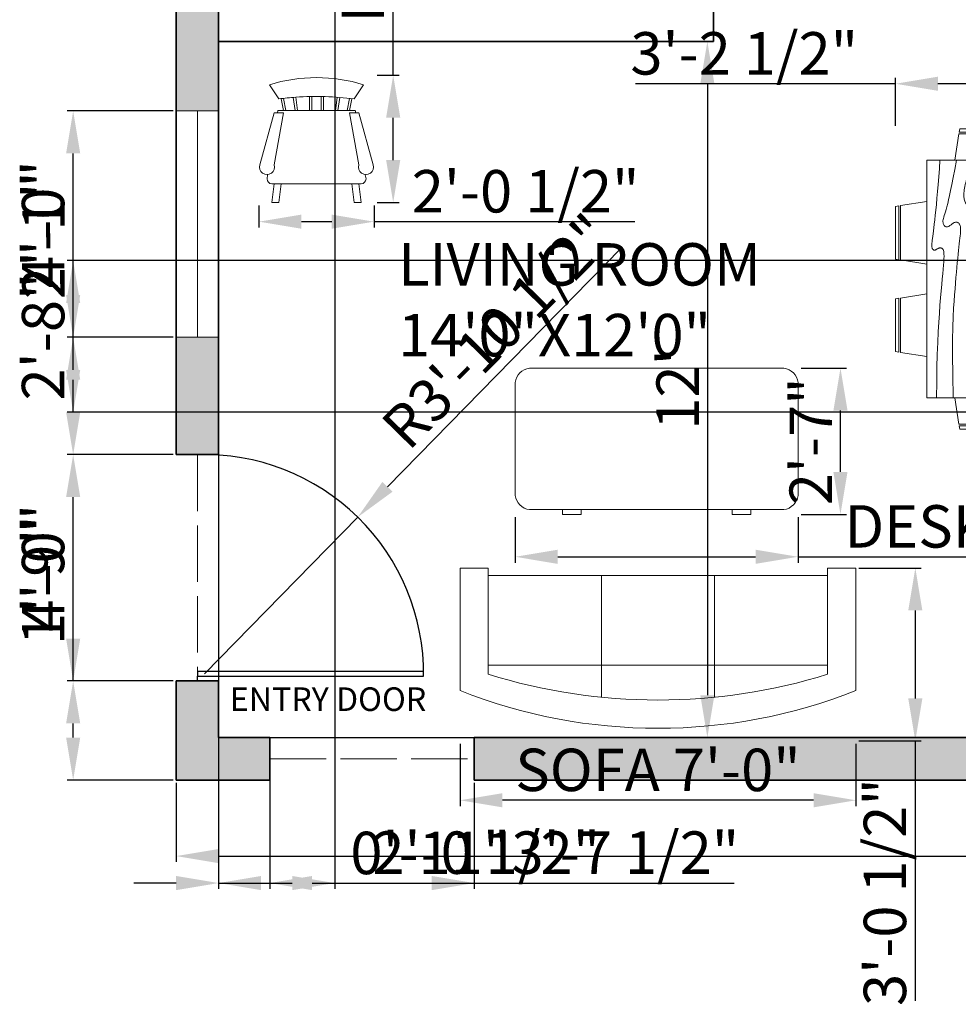
# Model space of a CAD drawing. Units: inches. Extents: x 39700 to 40173, y 40700 to 41139.
# Tile 1 of 4: x 39700 to 39899, y 40700 to 40909. Entities that reach past the tile are written whole.
import ezdxf

# ---------------------------------------------------------------- set-up
doc = ezdxf.new("R2010")
doc.units = ezdxf.units.IN
doc.linetypes.add('ACAD_ISO02W100', pattern=[15, 12, -3])
for name, color, linetype, lineweight in [('A-ANNO-DIMS', 2, 'Continuous', 18), ('A-ANNO-TEXT', 7, 'Continuous', 25), ('A-AREA-IDEN', 7, 'Continuous', 25), ('A-DOOR', 4, 'Continuous', 25), ('A-DOOR-HIDN', 4, 'ACAD_ISO02W100', 13), ('A-FURN', 8, 'Continuous', 18), ('A-GLAZ', 4, 'Continuous', 18), ('A-GLAZ-HIDN', 4, 'ACAD_ISO02W100', 13), ('A-WALL', 7, 'Continuous', 35)]:
    doc.layers.add(name, color=color, linetype=linetype, lineweight=lineweight)
doc.layers.add('A-WALL-PATT', color=251, linetype='Continuous', lineweight=13, true_color=0x636466)
doc.styles.get("Standard").update_dxf_attribs({"font": 'arial.ttf'})
doc.dimstyles.new('ISO-25', dxfattribs={"dimtxt": 9, "dimasz": 9, "dimexe": 1.25, "dimexo": 0.625, "dimtad": 1, "dimdec": 1, "dimrnd": 9, "dimlunit": 3, "dimtxsty": 'Standard', "dimcen": 2.5, "dimadec": 0, "dimazin": 0, "dimtfac": 1, "dimtdec": 1, "dimtmove": 0, "dimatfit": 3, "dimfxl": 1, "dimarcsym": 0})

# ---------------------------------------------------------------- blocks, each defined once
blk = doc.blocks.new('*D8')
at = {"layer": 'A-ANNO-DIMS', "color": 0, "lineweight": -2, "transparency": 16777216}
for p, q in [((39743.05, 40904.69), (39847.38, 40904.69)), ((39846.13, 40895.69), (39846.13, 40766.04)), ((39743.05, 40757.04), (39847.38, 40757.04))]:
    blk.add_line(p, q, dxfattribs=at)
at = {"layer": 'A-ANNO-DIMS', "color": 0, "transparency": 16777216}
for points in [[(39844.63, 40895.69), (39847.63, 40895.69), (39846.13, 40904.69)], [(39844.63, 40766.04), (39847.63, 40766.04), (39846.13, 40757.04)]]:
    blk.add_solid(points, dxfattribs=at)
at = {"layer": 'Defpoints', "color": 0, "transparency": 16777216}
for p in [(39742.42, 40904.69), (39742.42, 40757.04), (39846.13, 40757.04)]:
    blk.add_point(p, dxfattribs=at)
at = {"layer": 'A-ANNO-DIMS', "color": 0, "transparency": 16777216, "insert": (39840.99, 40830.87), "char_height": 9, "attachment_point": 5, "rotation": 90}
blk.add_mtext("12'", dxfattribs=at)
blk = doc.blocks.new('Dining Set - 36 x 72 in.')
for p, q in [((-22, 27.5), (-22.1562, 26.50042)), ((-22, 27.5), (-6, 27.5)), ((-5.8437, 26.49966), (-6, 27.5)), ((6, 27.5), (5.8438, 26.50042)), ((6, 27.5), (22, 27.5)), ((22.1563, 26.49966), (22, 27.5)), ((-22.2343, 26.00059), (-23.4847, 17.99762)), ((-22.2304, 26), (-5.7608, 26)), ((-5.8416, 26.5), (-22.1534, 26.5)), ((-4.5152, 17.99762), (-5.7655, 25.99926)), ((5.7657, 26.00059), (4.5153, 17.99762)), ((5.7696, 26), (22.2392, 26)), ((22.1584, 26.5), (5.8466, 26.5)), ((23.4848, 17.99762), (22.2345, 25.99926)), ((36, 18), (-36, 18)), ((-36, 18), (-36, -18)), ((36, -18), (36, 18)), ((-44.0006, 8.23428), (-35.9976, 9.48474)), ((44.0006, 8.23428), (35.9976, 9.48474)), ((-45.5, 8), (-44.5004, 8.15617)), ((-45.5, 8), (-45.5, -8)), ((-44.5, -8.15843), (-44.5, 8.15338)), ((-44, 8.23041), (-44, -8.23915)), ((44, 8.23041), (44, -8.23915)), ((44.5, -8.15843), (44.5, 8.15338)), ((45.5, 8), (44.5005, 8.15617)), ((45.5, 8), (45.5, -8)), ((-44.4997, -8.15631), (-45.5, -8)), ((-35.9976, -9.48476), (-43.9993, -8.2345)), ((35.9976, -9.48476), (43.9993, -8.2345)), ((44.4997, -8.15631), (45.5, -8)), ((-36, -18), (36, -18)), ((-22.2343, -26.0006), (-23.4847, -17.99762)), ((-4.5152, -17.99762), (-5.7655, -25.99928)), ((5.7657, -26.0006), (4.5153, -17.99762)), ((23.4848, -17.99762), (22.2345, -25.99928)), ((-22.2304, -26), (-5.7608, -26)), ((-22, -27.5), (-22.1562, -26.50044)), ((-5.8416, -26.5), (-22.1534, -26.5)), ((-5.8437, -26.49967), (-6, -27.5)), ((5.7696, -26), (22.2392, -26)), ((6, -27.5), (5.8438, -26.50044)), ((22.1584, -26.5), (5.8466, -26.5)), ((22.1563, -26.49967), (22, -27.5)), ((-22, -27.5), (-6, -27.5)), ((6, -27.5), (22, -27.5))]:
    blk.add_line(p, q)
for points in [[(-36, 15), (-31.1772, 14.97754), (-26.8079, 14.91406), (-22.8538, 14.81543), (-19.276, 14.6875), (-16.0362, 14.53613), (-13.0957, 14.36718), (-10.4159, 14.18652), (-7.9583, 14), (-5.6904, 13.81315), (-3.6035, 13.63021), (-1.6954, 13.45508), (0.0365, 13.29166), (1.5945, 13.14388), (2.9811, 13.01562), (4.1988, 12.9108), (5.25, 12.83333), (6.1393, 12.78613), (6.8802, 12.76823), (7.4883, 12.77767), (7.9792, 12.8125), (8.3685, 12.87077), (8.6719, 12.95052), (8.9049, 13.0498), (9.0833, 13.16666), (9.2205, 13.29899), (9.3216, 13.44401), (9.3895, 13.59879), (9.4271, 13.76041), (9.4373, 13.92594), (9.4232, 14.09245), (9.3875, 14.257), (9.3333, 14.41666), (9.2638, 14.56917), (9.1836, 14.71484), (9.0975, 14.85465), (9.0104, 14.98958), (8.9272, 15.1206), (8.8529, 15.2487), (8.7922, 15.37483), (8.75, 15.5), (8.7305, 15.62467), (8.7344, 15.74739), (8.7617, 15.86621), (8.8125, 15.97916), (8.8867, 16.08431), (8.9844, 16.17968), (9.1055, 16.26334), (9.25, 16.33333), (9.4189, 16.38802), (9.6172, 16.42708), (9.8506, 16.45052), (10.125, 16.45833), (10.4463, 16.45052), (10.8203, 16.42708), (11.2529, 16.38802), (11.75, 16.33333), (12.3184, 16.26318), (12.9694, 16.17838), (13.7151, 16.07991), (14.5677, 15.96875), (15.5395, 15.84586), (16.6426, 15.71224), (17.8893, 15.56884), (19.2917, 15.41666), (20.859, 15.25667), (22.5879, 15.08984), (24.4721, 14.91715), (26.5052, 14.73958), (28.6809, 14.5581), (30.9929, 14.3737), (33.4347, 14.18733), (36, 14)], [(-36, 10), (-28.9766, 10.14274), (-23.1725, 10.20442), (-18.4241, 10.19775), (-14.5677, 10.13541), (-11.4399, 10.03011), (-8.877, 9.89453), (-6.7154, 9.74137), (-4.7917, 9.58333), (-2.9698, 9.43082), (-1.2246, 9.28515), (0.4415, 9.14534), (2.026, 9.01041), (3.5266, 8.87939), (4.9408, 8.7513), (6.266, 8.62516), (7.5, 8.5), (8.6411, 8.37549), (9.6914, 8.2539), (10.6538, 8.13818), (11.5312, 8.03125), (12.3267, 7.93603), (13.043, 7.85547), (13.6831, 7.79248), (14.25, 7.75), (14.7471, 7.7303), (15.1797, 7.73307), (15.5537, 7.75732), (15.875, 7.80208), (16.1494, 7.86637), (16.3828, 7.94922), (16.5811, 8.04964), (16.75, 8.16666), (16.8944, 8.29915), (17.0143, 8.44531), (17.1089, 8.60319), (17.1771, 8.77083), (17.218, 8.94629), (17.2305, 9.1276), (17.2137, 9.31282), (17.1667, 9.5), (17.0895, 9.6875), (16.987, 9.875), (16.8649, 10.0625), (16.7292, 10.25), (16.5856, 10.4375), (16.4401, 10.625), (16.2985, 10.8125), (16.1667, 11), (16.05, 11.18733), (15.9518, 11.3737), (15.8752, 11.5581), (15.8229, 11.73958), (15.798, 11.91715), (15.8034, 12.08984), (15.842, 12.25667), (15.9167, 12.41666), (16.0295, 12.56836), (16.1784, 12.70833), (16.3605, 12.83268), (16.5729, 12.9375), (16.8127, 13.01888), (17.0768, 13.07291), (17.3625, 13.0957), (17.6667, 13.08333), (17.9894, 13.03312), (18.3418, 12.94726), (18.7382, 12.82918), (19.1927, 12.68229), (19.7195, 12.51001), (20.3327, 12.31575), (21.0465, 12.10294), (21.875, 11.875), (22.8357, 11.63354), (23.959, 11.37304), (25.2786, 11.08618), (26.8282, 10.76562), (28.6414, 10.40405), (30.752, 9.99414), (33.1936, 9.52856), (36, 9)], [(-36, 5.5), (-30.7157, 5.3348), (-26.069, 5.20963), (-21.9946, 5.11767), (-18.4271, 5.05208), (-15.3009, 5.00602), (-12.5508, 4.97265), (-10.1112, 4.94515), (-7.9167, 4.91666), (-5.909, 4.88167), (-4.0586, 4.83984), (-2.3429, 4.79215), (-0.7396, 4.73958), (0.7739, 4.6831), (2.22, 4.6237), (3.6213, 4.56233), (5, 4.5), (6.373, 4.43782), (7.7344, 4.3776), (9.0723, 4.32129), (10.375, 4.27083), (11.6309, 4.22819), (12.8281, 4.19531), (13.9551, 4.17415), (15, 4.16666), (15.954, 4.17448), (16.819, 4.19791), (17.6001, 4.23698), (18.3021, 4.29166), (18.9299, 4.36198), (19.4883, 4.44791), (19.9823, 4.54948), (20.4167, 4.66666), (20.7969, 4.79899), (21.1302, 4.94401), (21.4245, 5.09879), (21.6875, 5.26041), (21.9271, 5.42594), (22.1511, 5.59245), (22.3672, 5.757), (22.5834, 5.91666), (22.8065, 6.06868), (23.0404, 6.21093), (23.2879, 6.34147), (23.5521, 6.45833), (23.8358, 6.55957), (24.142, 6.64323), (24.4735, 6.70735), (24.8334, 6.75), (25.2235, 6.76969), (25.642, 6.76692), (26.0858, 6.74267), (26.5521, 6.69791), (27.0379, 6.63362), (27.5404, 6.55078), (28.0565, 6.45036), (28.5834, 6.33333), (29.1242, 6.19987), (29.7071, 6.04687), (30.3661, 5.87044), (31.1354, 5.66666), (32.0493, 5.43164), (33.142, 5.16146), (34.4475, 4.85221), (36, 4.5)], [(-36, -1), (-30.7915, -0.6591), (-26.0195, -0.38216), (-21.6519, -0.16284), (-17.6563, 0.00521), (-14.0005, 0.12833), (-10.6523, 0.21289), (-7.5796, 0.26522), (-4.75, 0.29166), (-2.134, 0.29793), (0.2878, 0.28711), (2.5317, 0.26163), (4.6146, 0.22396), (6.5529, 0.17651), (8.3633, 0.12174), (10.0623, 0.06209), (11.6667, 0), (13.1899, -0.06201), (14.6341, -0.1211), (15.9982, -0.17432), (17.2813, -0.21875), (18.4823, -0.25147), (19.6003, -0.26953), (20.6343, -0.27002), (21.5834, -0.25), (22.4481, -0.20768), (23.2357, -0.14584), (23.9549, -0.06836), (24.6146, 0.02083), (25.2235, 0.11784), (25.7904, 0.21875), (26.3241, 0.31966), (26.8334, 0.41666), (27.3265, 0.50618), (27.8099, 0.58593), (28.2894, 0.65397), (28.7709, 0.70833), (29.2601, 0.74707), (29.763, 0.76823), (30.2855, 0.76985), (30.8334, 0.75), (31.4088, 0.70784), (31.9994, 0.64713), (32.589, 0.57275), (33.1615, 0.48958), (33.7008, 0.4025), (34.1908, 0.3164), (34.6153, 0.23616), (34.9584, 0.16666), (35.2099, 0.11165), (35.3848, 0.07031), (35.504, 0.04069), (35.5886, 0.02083), (35.6594, 0.00879), (35.7377, 0.0026), (35.8442, 0.00032), (36, 0)], [(-36, -6.5), (-27.1843, -6.31267), (-20.084, -6.1263), (-14.469, -5.9419), (-10.1094, -5.76042), (-6.7752, -5.58285), (-4.2363, -5.41016), (-2.2629, -5.24333), (-0.625, -5.08334), (0.8708, -4.93099), (2.2715, -4.78646), (3.5872, -4.64974), (4.8281, -4.52084), (6.0046, -4.39974), (7.127, -4.28646), (8.2053, -4.18099), (9.25, -4.08334), (10.2705, -3.99382), (11.2734, -3.91407), (12.2647, -3.84603), (13.25, -3.79167), (14.2354, -3.75293), (15.2266, -3.73177), (16.2295, -3.73015), (17.25, -3.75), (18.2912, -3.79248), (19.3451, -3.85547), (20.4009, -3.93604), (21.4479, -4.03125), (22.4754, -4.13819), (23.4727, -4.25391), (24.4289, -4.37549), (25.3334, -4.5), (26.1785, -4.62492), (26.9694, -4.74935), (27.7145, -4.87281), (28.4219, -4.99479), (29.1, -5.11483), (29.7572, -5.23242), (30.4016, -5.34709), (31.0417, -5.45834), (31.6837, -5.56437), (32.3262, -5.65821), (32.9658, -5.73153), (33.599, -5.77604), (34.2224, -5.78345), (34.8327, -5.74545), (35.4264, -5.65373), (36, -5.5)], [(-36, -10), (-26.4022, -9.81299), (-18.4675, -9.62891), (-11.9839, -9.45069), (-6.7396, -9.28125), (-2.5226, -9.12354), (0.8789, -8.98047), (3.6769, -8.85498), (6.0833, -8.75), (8.2767, -8.66765), (10.3021, -8.60677), (12.1712, -8.56543), (13.8958, -8.54167), (15.4876, -8.53353), (16.9583, -8.53907), (18.3197, -8.55632), (19.5834, -8.58334), (20.7616, -8.61841), (21.8685, -8.66081), (22.9188, -8.71004), (23.9271, -8.76563), (24.9081, -8.82707), (25.8763, -8.89388), (26.8465, -8.96558), (27.8334, -9.04167), (28.8474, -9.12118), (29.8828, -9.20117), (30.93, -9.27824), (31.9792, -9.34896), (33.0205, -9.40991), (34.0443, -9.45768), (35.0407, -9.48885), (36, -9.5)], [(-36, -14.5), (-30.0881, -14.33513), (-25.0332, -14.21224), (-20.7312, -14.12647), (-17.0781, -14.07292), (-13.97, -14.04671), (-11.3027, -14.04297), (-8.9724, -14.05681), (-6.875, -14.08334), (-4.9224, -14.11833), (-3.0905, -14.16016), (-1.3709, -14.20785), (0.2448, -14.26042), (1.7647, -14.3169), (3.1973, -14.3763), (4.5507, -14.43767), (5.8333, -14.5), (7.0554, -14.5621), (8.235, -14.62175), (9.3922, -14.67652), (10.5469, -14.72396), (11.7192, -14.76164), (12.929, -14.78711), (14.1965, -14.79794), (15.5417, -14.79167), (16.9933, -14.76424), (18.6152, -14.70508), (20.4804, -14.60197), (22.6615, -14.44271), (25.2312, -14.21509), (28.2624, -13.9069), (31.8277, -13.50594), (36, -13)]]:
    blk.add_lwpolyline(points)
blk = doc.blocks.new('Sofa - Roundback 7 ft.')
for p, q in [((-12.00002, -32.4421), (-12.00003, -6.5971)), ((11.99997, -32.4421), (11.99998, -6.5971)), ((-36.000027, -34), (-36.000027, -11.4696)), ((35.99998, -34), (35.99998, -11.4696)), ((-35.999844, -13.3819), (35.9998, -13.3819)), ((-36.000027, -32.4421), (35.99998, -32.4421))]:
    blk.add_line(p, q)
for points in [[(-36.000027, -34), (-42.000027, -34), (-42.000027, -8)], [(41.99998, -8), (41.99998, -34), (35.99998, -34)]]:
    blk.add_lwpolyline(points)
for centre, radius, start, end in [((0, -114.25), 114.25, 68.43141, 111.5686), ((-0.00001, -127.1968), 121.1968, 72.72033, 107.2797)]:
    blk.add_arc(centre, radius, start, end)
blk = doc.blocks.new('Desk - 30 x 60 in.')
for p, q in [((-26.999995, 0), (26.999995, 0)), ((-29.999995, -27), (-29.999995, -3)), ((29.999995, -3), (29.999995, -27)), ((26.999995, -30), (-26.999995, -30)), ((-20.000005, -30), (-20.000005, -31)), ((-20.000005, -31), (-16.000005, -31)), ((-16.000005, -31), (-16.000005, -30)), ((15.999995, -31), (15.999995, -30)), ((19.999995, -31), (15.999995, -31)), ((19.999995, -30), (19.999995, -31))]:
    blk.add_line(p, q)
for centre, start, end in [((-26.499995, -3.5), 98.1301, 171.8699), ((26.499995, -3.5), 8.130102, 81.8699), ((-26.499995, -26.5), 188.1301, 261.8699), ((26.499995, -26.5), 278.1301, 351.8699)]:
    blk.add_arc(centre, 3.535534, start, end)
blk = doc.blocks.new('Chair - Rocking')
for p, q in [((-8, -4.5), (-10, -1.5)), ((8, -4.5), (10, -1.5)), ((-4, -7), (-4.40532, -4.16272)), ((-1.5, -4.05012), (-1.5, -7)), ((-1, -7), (-1, -4.05012)), ((1, -7), (1, -4.04655)), ((1.5, -4.05012), (1.5, -7)), ((-7.5, -4.5), (-7, -7)), ((-6.5, -7), (-7.02225, -4.43)), ((-4.5, -7), (-4.96674, -4.19951)), ((4, -7), (4.40187, -4.18694)), ((4.5, -7), (4.96761, -4.19437)), ((6.5, -7), (7, -4.4057)), ((7.5, -4.5), (7, -7)), ((-9, -7.5), (-12, -18.49999)), ((-7, -7.5), (-9, -7.5)), ((-9, -18.49999), (-7, -7.5)), ((-8.23428, -6.99939), (-8.3093, -7.47958)), ((-8.23041, -7), (8.23915, -7)), ((7, -7.5), (9, -7.5)), ((9, -18.49999), (7, -7.5)), ((8.31071, -7.48854), (8.23449, -7.00073)), ((9, -7.5), (12, -18.49999)), ((-10.36644, -20.64523), (-10.5, -21.49999)), ((10.5, -21.49999), (10.3575, -20.58798)), ((-9, -22.49999), (-9.5, -26.49999)), ((0, -22.49999), (-9.5, -22.49999)), ((-8, -26.49999), (-7.5, -22.49999)), ((0, -22.49999), (9.5, -22.49999)), ((8, -26.49999), (7.5, -22.49999)), ((9, -22.49999), (9.5, -26.49999)), ((-9.5, -26.49999), (-8, -26.49999)), ((9.5, -26.49999), (8, -26.49999))]:
    blk.add_line(p, q)
for centre, radius, start, end in [((0, -34.08333), 34.08333, 72.93847, 107.0615), ((0, -68.25004), 64.25, 93.92211, 97.15267), ((0, -68.25004), 64.25, 82.84733, 93.92211), ((-10.5, -18.99999), 1.58114, 161.5651, 18.43495), ((10.5, -18.99999), 1.58114, 161.5651, 18.43495), ((-9.5, -21.49999), 1, 180, 270), ((9.5, -21.49999), 1, 270, 0)]:
    blk.add_arc(centre, radius, start, end)
blk = doc.blocks.new('*D21')
at = {"layer": 'A-ANNO-DIMS', "color": 0, "lineweight": -2, "transparency": 16777216}
for p, q in [((39733.42, 40747.42), (39733.42, 40730.66)), ((40093.42, 40747.42), (40093.42, 40730.66)), ((39742.42, 40731.91), (40084.42, 40731.91))]:
    blk.add_line(p, q, dxfattribs=at)
at = {"layer": 'A-ANNO-DIMS', "color": 0, "transparency": 16777216}
for points in [[(39742.42, 40733.41), (39742.42, 40730.41), (39733.42, 40731.91)], [(40084.42, 40733.41), (40084.42, 40730.41), (40093.42, 40731.91)]]:
    blk.add_solid(points, dxfattribs=at)
at = {"layer": 'Defpoints', "color": 0, "transparency": 16777216}
for p in [(39733.42, 40748.04), (40093.42, 40748.04), (40093.42, 40731.91)]:
    blk.add_point(p, dxfattribs=at)
at = {"layer": 'A-ANNO-DIMS', "color": 0, "transparency": 16777216, "insert": (39913.42, 40737.13), "char_height": 9, "attachment_point": 5}
blk.add_mtext("30'", dxfattribs=at)
blk = doc.blocks.new('*D31')
at = {"layer": 'A-ANNO-DIMS', "color": 0, "lineweight": -2, "transparency": 16777216}
for p, q in [((39886.03, 40886.79), (39886.03, 40896.97)), ((39924.53, 40886.79), (39924.53, 40896.97)), ((39886.03, 40895.72), (39830.89, 40895.72)), ((39915.53, 40895.72), (39895.03, 40895.72))]:
    blk.add_line(p, q, dxfattribs=at)
at = {"layer": 'A-ANNO-DIMS', "color": 0, "transparency": 16777216}
for points in [[(39895.03, 40897.22), (39895.03, 40894.22), (39886.03, 40895.72)], [(39915.53, 40897.22), (39915.53, 40894.22), (39924.53, 40895.72)]]:
    blk.add_solid(points, dxfattribs=at)
at = {"layer": 'Defpoints', "color": 0, "transparency": 16777216}
for p in [(39886.03, 40895.72), (39886.03, 40886.16), (39924.53, 40886.16)]:
    blk.add_point(p, dxfattribs=at)
at = {"layer": 'A-ANNO-DIMS', "color": 0, "transparency": 16777216, "insert": (39853.96, 40901), "char_height": 9, "attachment_point": 5}
blk.add_mtext('3\'-2 1/2"', dxfattribs=at)
blk = doc.blocks.new('*D32')
at = {"layer": 'A-ANNO-DIMS', "color": 0, "lineweight": -2, "transparency": 16777216}
for p, q in [((39793.65, 40755.72), (39793.65, 40742.5)), ((39877.65, 40755.72), (39877.65, 40742.5)), ((39868.65, 40743.75), (39802.65, 40743.75))]:
    blk.add_line(p, q, dxfattribs=at)
at = {"layer": 'A-ANNO-DIMS', "color": 0, "transparency": 16777216}
for points in [[(39802.65, 40745.25), (39802.65, 40742.25), (39793.65, 40743.75)], [(39868.65, 40745.25), (39868.65, 40742.25), (39877.65, 40743.75)]]:
    blk.add_solid(points, dxfattribs=at)
at = {"layer": 'Defpoints', "color": 0, "transparency": 16777216}
for p in [(39793.65, 40756.35), (39877.65, 40756.35), (39793.65, 40743.75)]:
    blk.add_point(p, dxfattribs=at)
at = {"layer": 'A-ANNO-DIMS', "color": 0, "transparency": 16777216, "insert": (39835.65, 40749.03), "char_height": 9, "attachment_point": 5}
blk.add_mtext('SOFA 7\'-0"', dxfattribs=at)
blk = doc.blocks.new('*D33')
at = {"layer": 'A-ANNO-DIMS', "color": 0, "lineweight": -2, "transparency": 16777216}
for p, q in [((39878.28, 40793.01), (39891.5, 40793.01)), ((39890.25, 40784.01), (39890.25, 40765.35)), ((39878.28, 40756.35), (39891.5, 40756.35)), ((39890.25, 40756.35), (39890.25, 40701.21))]:
    blk.add_line(p, q, dxfattribs=at)
at = {"layer": 'A-ANNO-DIMS', "color": 0, "transparency": 16777216}
for points in [[(39888.75, 40784.01), (39891.75, 40784.01), (39890.25, 40793.01)], [(39888.75, 40765.35), (39891.75, 40765.35), (39890.25, 40756.35)]]:
    blk.add_solid(points, dxfattribs=at)
at = {"layer": 'Defpoints', "color": 0, "transparency": 16777216}
for p in [(39877.65, 40793.01), (39877.65, 40756.35), (39890.25, 40756.35)]:
    blk.add_point(p, dxfattribs=at)
at = {"layer": 'A-ANNO-DIMS', "color": 0, "transparency": 16777216, "insert": (39884.97, 40724.28), "char_height": 9, "attachment_point": 5, "rotation": 90}
blk.add_mtext('3\'-0 1/2"', dxfattribs=at)
blk = doc.blocks.new('*D34')
at = {"layer": 'A-ANNO-DIMS', "color": 0, "lineweight": -2, "transparency": 16777216}
for p, q in [((39805.37, 40803.76), (39805.37, 40794.14)), ((39865.37, 40803.76), (39865.37, 40794.14)), ((39814.37, 40795.39), (39856.37, 40795.39)), ((39865.37, 40795.39), (39936.83, 40795.39))]:
    blk.add_line(p, q, dxfattribs=at)
at = {"layer": 'A-ANNO-DIMS', "color": 0, "transparency": 16777216}
for points in [[(39814.37, 40796.89), (39814.37, 40793.89), (39805.37, 40795.39)], [(39856.37, 40796.89), (39856.37, 40793.89), (39865.37, 40795.39)]]:
    blk.add_solid(points, dxfattribs=at)
at = {"layer": 'Defpoints', "color": 0, "transparency": 16777216}
for p in [(39805.37, 40804.39), (39865.37, 40804.39), (39865.37, 40795.39)]:
    blk.add_point(p, dxfattribs=at)
at = {"layer": 'A-ANNO-DIMS', "color": 0, "transparency": 16777216, "insert": (39905.6, 40800.67), "char_height": 9, "attachment_point": 5}
blk.add_mtext('DESK 5\'-0"', dxfattribs=at)
blk = doc.blocks.new('*D35')
at = {"layer": 'A-ANNO-DIMS', "color": 0, "lineweight": -2, "transparency": 16777216}
for p, q in [((39866, 40835.39), (39875.62, 40835.39)), ((39874.37, 40813.39), (39874.37, 40826.39)), ((39866, 40804.39), (39875.62, 40804.39))]:
    blk.add_line(p, q, dxfattribs=at)
at = {"layer": 'A-ANNO-DIMS', "color": 0, "transparency": 16777216}
for points in [[(39872.87, 40826.39), (39875.87, 40826.39), (39874.37, 40835.39)], [(39872.87, 40813.39), (39875.87, 40813.39), (39874.37, 40804.39)]]:
    blk.add_solid(points, dxfattribs=at)
at = {"layer": 'Defpoints', "color": 0, "transparency": 16777216}
for p in [(39865.37, 40835.39), (39874.37, 40835.39), (39865.37, 40804.39)]:
    blk.add_point(p, dxfattribs=at)
at = {"layer": 'A-ANNO-DIMS', "color": 0, "transparency": 16777216, "insert": (39869.23, 40819.89), "char_height": 9, "attachment_point": 5, "rotation": 90}
blk.add_mtext('2\'-7"', dxfattribs=at)
blk = doc.blocks.new('*D36')
at = {"layer": 'A-ANNO-DIMS', "color": 0, "lineweight": -2, "transparency": 16777216}
for p, q in [((39779.47, 40897.52), (39779.47, 40988.51)), ((39776.04, 40897.52), (39780.72, 40897.52)), ((39779.47, 40879.52), (39779.47, 40888.52)), ((39776.04, 40870.52), (39780.72, 40870.52))]:
    blk.add_line(p, q, dxfattribs=at)
at = {"layer": 'A-ANNO-DIMS', "color": 0, "transparency": 16777216}
for points in [[(39777.97, 40888.52), (39780.97, 40888.52), (39779.47, 40897.52)], [(39777.97, 40879.52), (39780.97, 40879.52), (39779.47, 40870.52)]]:
    blk.add_solid(points, dxfattribs=at)
at = {"layer": 'Defpoints', "color": 0, "transparency": 16777216}
for p in [(39775.42, 40897.52), (39779.47, 40897.52), (39775.42, 40870.52)]:
    blk.add_point(p, dxfattribs=at)
at = {"layer": 'A-ANNO-DIMS', "color": 0, "transparency": 16777216, "insert": (39774.18, 40947.51), "char_height": 9, "attachment_point": 5, "rotation": 90}
blk.add_mtext('ROCKER 2\'-3"', dxfattribs=at)
blk = doc.blocks.new('*D37')
at = {"layer": 'A-ANNO-DIMS', "color": 0, "lineweight": -2, "transparency": 16777216}
for p, q in [((39750.98, 40869.89), (39750.98, 40865.22)), ((39775.42, 40869.89), (39775.42, 40865.22)), ((39759.98, 40866.47), (39766.42, 40866.47)), ((39775.42, 40866.47), (39830.72, 40866.47))]:
    blk.add_line(p, q, dxfattribs=at)
at = {"layer": 'A-ANNO-DIMS', "color": 0, "transparency": 16777216}
for points in [[(39759.98, 40867.97), (39759.98, 40864.97), (39750.98, 40866.47)], [(39766.42, 40867.97), (39766.42, 40864.97), (39775.42, 40866.47)]]:
    blk.add_solid(points, dxfattribs=at)
at = {"layer": 'Defpoints', "color": 0, "transparency": 16777216}
for p in [(39750.98, 40870.52), (39775.42, 40870.52), (39775.42, 40866.47)]:
    blk.add_point(p, dxfattribs=at)
at = {"layer": 'A-ANNO-DIMS', "color": 0, "transparency": 16777216, "insert": (39807.57, 40871.75), "char_height": 9, "attachment_point": 5}
blk.add_mtext('2\'-0 1/2"', dxfattribs=at)
blk = doc.blocks.new('*D40')
at = {"layer": 'A-ANNO-DIMS', "color": 0, "lineweight": -2, "transparency": 16777216}
for p, q in [((39711.57, 40769.06), (39711.57, 40802.39)), ((39732.8, 40769.06), (39710.32, 40769.06)), ((39711.57, 40757.04), (39711.57, 40760.06)), ((39732.8, 40748.04), (39710.32, 40748.04))]:
    blk.add_line(p, q, dxfattribs=at)
at = {"layer": 'A-ANNO-DIMS', "color": 0, "transparency": 16777216}
for points in [[(39710.07, 40760.06), (39713.07, 40760.06), (39711.57, 40769.06)], [(39710.07, 40757.04), (39713.07, 40757.04), (39711.57, 40748.04)]]:
    blk.add_solid(points, dxfattribs=at)
at = {"layer": 'Defpoints', "color": 0, "transparency": 16777216}
for p in [(39711.57, 40769.06), (39733.42, 40769.06), (39733.42, 40748.04)]:
    blk.add_point(p, dxfattribs=at)
at = {"layer": 'A-ANNO-DIMS', "color": 0, "transparency": 16777216, "insert": (39706.35, 40790.23), "char_height": 9, "attachment_point": 5, "rotation": 90}
blk.add_mtext('1\'-9"', dxfattribs=at)
blk = doc.blocks.new('*D41')
at = {"layer": 'A-ANNO-DIMS', "color": 0, "lineweight": -2, "transparency": 16777216}
for p, q in [((39732.8, 40817.06), (39710.32, 40817.06)), ((39711.57, 40778.06), (39711.57, 40808.06)), ((39732.8, 40769.06), (39710.32, 40769.06))]:
    blk.add_line(p, q, dxfattribs=at)
at = {"layer": 'A-ANNO-DIMS', "color": 0, "transparency": 16777216}
for points in [[(39710.07, 40808.06), (39713.07, 40808.06), (39711.57, 40817.06)], [(39710.07, 40778.06), (39713.07, 40778.06), (39711.57, 40769.06)]]:
    blk.add_solid(points, dxfattribs=at)
at = {"layer": 'Defpoints', "color": 0, "transparency": 16777216}
for p in [(39711.57, 40817.06), (39733.42, 40817.06), (39733.42, 40769.06)]:
    blk.add_point(p, dxfattribs=at)
at = {"layer": 'A-ANNO-DIMS', "color": 0, "transparency": 16777216, "insert": (39706.35, 40793.06), "char_height": 9, "attachment_point": 5, "rotation": 90}
blk.add_mtext('4\'-0"', dxfattribs=at)
blk = doc.blocks.new('*D42')
at = {"layer": 'A-ANNO-DIMS', "color": 0, "lineweight": -2, "transparency": 16777216}
for p, q in [((39711.57, 40841.95), (39711.57, 40876.28)), ((39732.8, 40841.95), (39710.32, 40841.95)), ((39711.57, 40826.06), (39711.57, 40832.95)), ((39732.8, 40817.06), (39710.32, 40817.06))]:
    blk.add_line(p, q, dxfattribs=at)
at = {"layer": 'A-ANNO-DIMS', "color": 0, "transparency": 16777216}
for points in [[(39710.07, 40832.95), (39713.07, 40832.95), (39711.57, 40841.95)], [(39710.07, 40826.06), (39713.07, 40826.06), (39711.57, 40817.06)]]:
    blk.add_solid(points, dxfattribs=at)
at = {"layer": 'Defpoints', "color": 0, "transparency": 16777216}
for p in [(39711.57, 40841.95), (39733.42, 40841.95), (39733.42, 40817.06)]:
    blk.add_point(p, dxfattribs=at)
at = {"layer": 'A-ANNO-DIMS', "color": 0, "transparency": 16777216, "insert": (39706.43, 40863.61), "char_height": 9, "attachment_point": 5, "rotation": 90}
blk.add_mtext('2\'-1"', dxfattribs=at)
blk = doc.blocks.new('*D43')
at = {"layer": 'A-ANNO-DIMS', "color": 0, "lineweight": -2, "transparency": 16777216}
for p, q in [((39732.8, 40889.95), (39710.32, 40889.95)), ((39711.57, 40850.95), (39711.57, 40880.95)), ((39732.8, 40841.95), (39710.32, 40841.95))]:
    blk.add_line(p, q, dxfattribs=at)
at = {"layer": 'A-ANNO-DIMS', "color": 0, "transparency": 16777216}
for points in [[(39710.07, 40880.95), (39713.07, 40880.95), (39711.57, 40889.95)], [(39710.07, 40850.95), (39713.07, 40850.95), (39711.57, 40841.95)]]:
    blk.add_solid(points, dxfattribs=at)
at = {"layer": 'Defpoints', "color": 0, "transparency": 16777216}
for p in [(39711.57, 40889.95), (39733.42, 40889.95), (39733.42, 40841.95)]:
    blk.add_point(p, dxfattribs=at)
at = {"layer": 'A-ANNO-DIMS', "color": 0, "transparency": 16777216, "insert": (39706.35, 40865.95), "char_height": 9, "attachment_point": 5, "rotation": 90}
blk.add_mtext('4\'-0"', dxfattribs=at)
blk = doc.blocks.new('*D44')
at = {"layer": 'A-ANNO-DIMS', "color": 0, "lineweight": -2, "transparency": 16777216}
for p, q in [((39742.42, 40756.42), (39742.42, 40724.94)), ((39753.27, 40756.42), (39753.27, 40724.94)), ((39733.42, 40726.19), (39724.42, 40726.19)), ((39742.42, 40726.19), (39753.27, 40726.19)), ((39762.27, 40726.19), (39803.43, 40726.19))]:
    blk.add_line(p, q, dxfattribs=at)
at = {"layer": 'A-ANNO-DIMS', "color": 0, "transparency": 16777216}
for points in [[(39733.42, 40727.69), (39733.42, 40724.69), (39742.42, 40726.19)], [(39762.27, 40727.69), (39762.27, 40724.69), (39753.27, 40726.19)]]:
    blk.add_solid(points, dxfattribs=at)
at = {"layer": 'Defpoints', "color": 0, "transparency": 16777216}
for p in [(39742.42, 40757.04), (39753.27, 40757.04), (39753.27, 40726.19)]:
    blk.add_point(p, dxfattribs=at)
at = {"layer": 'A-ANNO-DIMS', "color": 0, "transparency": 16777216, "insert": (39787.35, 40731.41), "char_height": 9, "attachment_point": 5}
blk.add_mtext('0\'-11"', dxfattribs=at)
blk = doc.blocks.new('*D45')
at = {"layer": 'A-ANNO-DIMS', "color": 0, "lineweight": -2, "transparency": 16777216}
for p, q in [((39753.27, 40747.42), (39753.27, 40724.94)), ((39796.66, 40747.42), (39796.66, 40724.94)), ((39762.27, 40726.19), (39787.66, 40726.19)), ((39796.66, 40726.19), (39851.8, 40726.19))]:
    blk.add_line(p, q, dxfattribs=at)
at = {"layer": 'A-ANNO-DIMS', "color": 0, "transparency": 16777216}
for points in [[(39762.27, 40727.69), (39762.27, 40724.69), (39753.27, 40726.19)], [(39787.66, 40727.69), (39787.66, 40724.69), (39796.66, 40726.19)]]:
    blk.add_solid(points, dxfattribs=at)
at = {"layer": 'Defpoints', "color": 0, "transparency": 16777216}
for p in [(39753.27, 40748.04), (39796.66, 40748.04), (39796.66, 40726.19)]:
    blk.add_point(p, dxfattribs=at)
at = {"layer": 'A-ANNO-DIMS', "color": 0, "transparency": 16777216, "insert": (39828.73, 40731.48), "char_height": 9, "attachment_point": 5}
blk.add_mtext('3\'-7 1/2"', dxfattribs=at)
blk = doc.blocks.new('*D48')
at = {"layer": 'A-ANNO-DIMS', "color": 0, "lineweight": -2, "transparency": 16777216}
for p, q in [((40043.02, 40858.21), (39710.32, 40858.21)), ((39711.57, 40835.04), (39711.57, 40849.21)), ((40043.02, 40826.04), (39710.32, 40826.04))]:
    blk.add_line(p, q, dxfattribs=at)
at = {"layer": 'A-ANNO-DIMS', "color": 0, "transparency": 16777216}
for points in [[(39710.07, 40849.21), (39713.07, 40849.21), (39711.57, 40858.21)], [(39710.07, 40835.04), (39713.07, 40835.04), (39711.57, 40826.04)]]:
    blk.add_solid(points, dxfattribs=at)
at = {"layer": 'Defpoints', "color": 0, "transparency": 16777216}
for p in [(39711.57, 40858.21), (40043.65, 40858.21), (40043.65, 40826.04)]:
    blk.add_point(p, dxfattribs=at)
at = {"layer": 'A-ANNO-DIMS', "color": 0, "transparency": 16777216, "insert": (39706.35, 40842.12), "char_height": 9, "attachment_point": 5, "rotation": 90}
blk.add_mtext('2\'-8"', dxfattribs=at)
blk = doc.blocks.new('*D49')
at = {"layer": 'A-ANNO-DIMS', "color": 0, "lineweight": -2, "transparency": 16777216}
for p, q in [((39742.42, 41013.67), (39742.42, 40724.94)), ((39767.06, 41013.67), (39767.06, 40724.94)), ((39751.42, 40726.19), (39758.06, 40726.19)), ((39767.06, 40726.19), (39822.36, 40726.19))]:
    blk.add_line(p, q, dxfattribs=at)
at = {"layer": 'A-ANNO-DIMS', "color": 0, "transparency": 16777216}
for points in [[(39751.42, 40727.69), (39751.42, 40724.69), (39742.42, 40726.19)], [(39758.06, 40727.69), (39758.06, 40724.69), (39767.06, 40726.19)]]:
    blk.add_solid(points, dxfattribs=at)
at = {"layer": 'Defpoints', "color": 0, "transparency": 16777216}
for p in [(39742.42, 41014.29), (39767.06, 41014.29), (39767.06, 40726.19)]:
    blk.add_point(p, dxfattribs=at)
at = {"layer": 'A-ANNO-DIMS', "color": 0, "transparency": 16777216, "insert": (39799.21, 40731.47), "char_height": 9, "attachment_point": 5}
blk.add_mtext('2\'-0 1/2"', dxfattribs=at)
blk = doc.blocks.new('*D52')
at = {"layer": 'A-ANNO-DIMS', "color": 0, "lineweight": -2, "transparency": 16777216}
for p, q in [((39827.75, 40860.79), (39778.25, 40810.24)), ((39739.4, 40770.56), (39771.95, 40803.8))]:
    blk.add_line(p, q, dxfattribs=at)
at = {"layer": 'A-ANNO-DIMS', "color": 0, "transparency": 16777216}
blk.add_solid([(39777.18, 40811.28), (39779.32, 40809.19), (39771.95, 40803.8)], dxfattribs=at)
at = {"layer": 'Defpoints', "color": 0, "transparency": 16777216}
for p in [(39771.95, 40803.8), (39739.4, 40770.56)]:
    blk.add_point(p, dxfattribs=at)
at = {"layer": 'A-ANNO-DIMS', "color": 0, "transparency": 16777216, "insert": (39802.37, 40842.42), "char_height": 9, "attachment_point": 5, "rotation": 45.6026}
blk.add_mtext('R3\'-10 1/2"', dxfattribs=at)

msp = doc.modelspace()

# ---------------------------------------------------------------- hatches: boundary and pattern name
at = {"layer": 'A-WALL-PATT'}
h = msp.add_hatch(color=256, dxfattribs=at)
h.dxf.hatch_style = 1
h.paths.add_polyline_path([(39742.42, 41039.04), (39838.42, 41039.04), (39838.42, 40943.28, -0.039113), (39842.92, 40942.53), (39847.42, 40942.53), (39847.42, 40946.04), (39850.1, 40946.04), (39850.1, 40955.04), (39847.42, 40955.04), (39847.42, 41039.04), (39895.42, 41039.04), (39895.42, 40955.04), (39874.1, 40955.04), (39874.1, 40951.54, -0.010637), (39874.1, 40950.54), (39874.1, 40946.04), (39895.42, 40946.04), (39904.42, 40946.04), (39904.42, 41039.04), (40084.42, 41039.04), (40084.42, 40895.04), (39960.51, 40895.04), (39960.51, 40886.04), (40084.42, 40886.04), (40084.42, 40817.04), (40093.42, 40817.04), (40093.42, 41048.04), (39733.42, 41048.04), (39733.42, 40889.95), (39742.42, 40889.95)])
h.paths.add_polyline_path([(39742.42, 40841.95), (39733.42, 40841.95), (39733.42, 40817.06), (39737.92, 40817.06, -0.015901), (39740.88, 40817.06), (39742.42, 40817.06)], flags=17)
h.paths.add_polyline_path([(40093.42, 40757.04), (39796.66, 40757.04), (39796.66, 40748.04), (40093.42, 40748.04)])
h.paths.add_polyline_path([(39753.27, 40757.04), (39742.42, 40757.04), (39742.42, 40769.06), (39733.42, 40769.06), (39733.42, 40748.04), (39753.27, 40748.04)])
h.paths.add_polyline_path([(40084.42, 40826.04), (39960.51, 40826.04), (39960.51, 40817.04), (40084.42, 40817.04)], flags=17)
h.paths.add_polyline_path([(39969.51, 40859.86), (39960.51, 40859.86), (39960.51, 40852.78), (39969.51, 40852.78)], flags=17)
h.paths.add_polyline_path([(39969.51, 40886.04), (39960.51, 40886.04), (39960.51, 40881.75), (39969.51, 40881.75)], flags=17)
h.paths.add_polyline_path([(39852.31, 40989.98), (39900.82, 40989.98), (39900.82, 41008.52), (39852.31, 41008.52)], flags=25)

# ---------------------------------------------------------------- linework, layer by layer
at = {"layer": 'A-DOOR'}
for p, q in [((39785.92, 40771.06), (39737.92, 40771.06)), ((39737.92, 40771.06), (39737.92, 40770.06)), ((39785.92, 40770.06), (39785.92, 40771.06)), ((39737.92, 40769.06), (39737.92, 40770.06)), ((39737.92, 40770.06), (39785.92, 40770.06))]:
    msp.add_line(p, q, dxfattribs=at)
msp.add_arc((39739.4, 40770.56), 46.52, 359.3842, 91.822, dxfattribs=at)
at = {"layer": 'A-DOOR-HIDN'}
msp.add_line((39737.92, 40817.06), (39737.92, 40769.56), dxfattribs=at)
at = {"layer": 'A-GLAZ'}
for p, q in [((39733.42, 40889.95), (39742.42, 40889.95)), ((39737.92, 40889.95), (39737.92, 40841.95)), ((39733.42, 40841.95), (39742.42, 40841.95))]:
    msp.add_line(p, q, dxfattribs=at)
at = {"layer": 'A-GLAZ-HIDN'}
msp.add_line((39753.27, 40752.54), (39796.66, 40752.54), dxfattribs=at)
at = {"layer": 'A-WALL'}
for p, q in [((39733.42, 41048.04), (39733.42, 40817.06)), ((39742.42, 41039.04), (39742.42, 40817.06)), ((39847.42, 40913.69), (39847.42, 40904.69)), ((39742.42, 40904.69), (39847.42, 40904.69)), ((39742.42, 40817.06), (39733.42, 40817.06)), ((39742.42, 40769.06), (39733.42, 40769.06)), ((39733.42, 40769.06), (39733.42, 40748.04)), ((39742.42, 40769.06), (39742.42, 40757.04)), ((39742.42, 40757.04), (39753.27, 40757.04)), ((39753.27, 40757.04), (39753.27, 40748.04)), ((39796.66, 40757.04), (39796.66, 40748.04)), ((39796.66, 40757.04), (40093.42, 40757.04)), ((39733.42, 40748.04), (39753.27, 40748.04)), ((39796.66, 40748.04), (40093.42, 40748.04))]:
    msp.add_line(p, q, dxfattribs=at)

# ---------------------------------------------------------------- block references
at = {"layer": 'A-FURN'}
for name, p in [('Chair - Rocking', (39763.2, 40897.02)), ('Desk - 30 x 60 in.', (39835.37, 40835.39))]:
    msp.add_blockref(name, p, dxfattribs=at)
at = {"layer": 'A-FURN', "xscale": 0.7, "yscale": 0.7, "rotation": 90}
msp.add_blockref('Dining Set - 36 x 72 in.', (39905.28, 40854.31), dxfattribs=at)
at = {"layer": 'A-FURN', "rotation": 180}
msp.add_blockref('Sofa - Roundback 7 ft.', (39835.65, 40759.01), dxfattribs=at)

# ---------------------------------------------------------------- texts
at = {"layer": 'A-ANNO-TEXT', "insert": (39744.82, 40767.69), "char_height": 5, "attachment_point": 1}
msp.add_mtext_dynamic_manual_height_columns('ENTRY DOOR', width=46.9136, gutter_width=12.5, heights=[0], dxfattribs=at)
at = {"layer": 'A-AREA-IDEN', "insert": (39780.51, 40861.91), "char_height": 9, "attachment_point": 1}
msp.add_mtext_dynamic_manual_height_columns('LIVING ROOM\\P14\'0"X12\'0"', width=87.8541, gutter_width=12.5, heights=[0], dxfattribs=at)

# ---------------------------------------------------------------- dimensions: what is measured, and where the dimension line sits
at = {"layer": 'A-ANNO-DIMS'}
for base, p1, p2, override, picture, middle in [((39767.06, 40726.19), (39742.42, 41014.29), (39767.06, 41014.29), {"dimdec": 1, "dimlfac": 1, "dimrnd": 0, "dimzin": 1, "dimdsep": 46, "dimlunit": 4, "dimfrac": 2}, '*D49', (39799.21, 40731.47)), ((39775.42, 40866.47), (39750.98, 40870.52), (39775.42, 40870.52), {"dimdec": 1, "dimlfac": 1, "dimrnd": 0, "dimzin": 1, "dimdsep": 46, "dimlunit": 4, "dimfrac": 2}, '*D37', (39807.57, 40871.75)), ((39753.2667, 40726.1943), (39742.4234, 40757.0443), (39753.2667, 40757.0443), {"dimdec": 1, "dimlfac": 1, "dimrnd": 0, "dimzin": 1, "dimdsep": 46, "dimlunit": 4, "dimfrac": 2}, '*D44', (39787.3501, 40731.4145)), ((40093.42, 40731.91), (39733.42, 40748.04), (40093.42, 40748.04), {"dimclrd": 0, "dimclre": 0, "dimclrt": 0}, '*D21', (39913.42, 40737.13)), ((39796.66, 40726.19), (39753.27, 40748.04), (39796.66, 40748.04), {"dimdec": 1, "dimlfac": 1, "dimrnd": 0, "dimzin": 1, "dimdsep": 46, "dimlunit": 4, "dimfrac": 2}, '*D45', (39828.73, 40731.48))]:
    dim = msp.add_linear_dim(base=base, p1=p1, p2=p2, dimstyle='ISO-25', override=override, dxfattribs=at)
    dim.commit()
    dim.dimension.update_dxf_attribs({"geometry": picture, "text_midpoint": middle})
for base, p1, p2, angle, text, picture, middle in [((39779.47, 40897.52), (39775.42, 40870.52), (39775.42, 40897.52), 90, 'ROCKER <>', '*D36', (39774.18, 40947.51)), ((39793.65, 40743.75), (39877.65, 40756.35), (39793.65, 40756.35), 180, 'SOFA <>', '*D32', (39835.65, 40749.03))]:
    dim = msp.add_linear_dim(base=base, p1=p1, p2=p2, angle=angle, text=text, dimstyle='ISO-25', override={"dimdec": 1, "dimlfac": 1, "dimrnd": 0, "dimzin": 1, "dimdsep": 46, "dimlunit": 4, "dimfrac": 2}, dxfattribs=at)
    dim.commit()
    dim.dimension.update_dxf_attribs({"geometry": picture, "text_midpoint": middle})
for base, p1, p2, angle, override, picture, middle in [((39886.03, 40895.72), (39924.53, 40886.16), (39886.03, 40886.16), 180, {"dimdec": 1, "dimlfac": 1, "dimrnd": 0, "dimzin": 1, "dimdsep": 46, "dimlunit": 4, "dimfrac": 2}, '*D31', (39853.96, 40901)), ((39846.132, 40757.0443), (39742.4234, 40904.6878), (39742.4234, 40757.0443), 90, {"dimclrd": 0, "dimclre": 0, "dimclrt": 0}, '*D8', (39840.9886, 40830.866)), ((39711.57, 40889.95), (39733.42, 40841.95), (39733.42, 40889.95), 90, {"dimdec": 1, "dimlfac": 1, "dimrnd": 0, "dimzin": 1, "dimdsep": 46, "dimlunit": 4, "dimfrac": 2}, '*D43', (39706.35, 40865.95)), ((39711.57, 40841.95), (39733.42, 40817.06), (39733.42, 40841.95), 90, {"dimdec": 1, "dimlfac": 1, "dimrnd": 0, "dimzin": 1, "dimdsep": 46, "dimlunit": 4, "dimfrac": 2}, '*D42', (39706.43, 40863.61)), ((39711.57, 40858.21), (40043.65, 40826.04), (40043.65, 40858.21), 90, {"dimdec": 1, "dimlfac": 1, "dimrnd": 0, "dimzin": 1, "dimdsep": 46, "dimlunit": 4, "dimfrac": 2}, '*D48', (39706.35, 40842.12)), ((39874.37, 40835.39), (39865.37, 40804.39), (39865.37, 40835.39), 90, {"dimdec": 1, "dimlfac": 1, "dimrnd": 0, "dimzin": 1, "dimdsep": 46, "dimlunit": 4, "dimfrac": 2}, '*D35', (39869.23, 40819.89)), ((39711.57, 40817.06), (39733.42, 40769.06), (39733.42, 40817.06), 90, {"dimdec": 1, "dimlfac": 1, "dimrnd": 0, "dimzin": 1, "dimdsep": 46, "dimlunit": 4, "dimfrac": 2}, '*D41', (39706.35, 40793.06)), ((39711.57, 40769.06), (39733.42, 40748.04), (39733.42, 40769.06), 90, {"dimdec": 1, "dimlfac": 1, "dimrnd": 0, "dimzin": 1, "dimdsep": 46, "dimlunit": 4, "dimfrac": 2}, '*D40', (39706.35, 40790.23)), ((39890.25, 40756.35), (39877.65, 40793.01), (39877.65, 40756.35), 270, {"dimdec": 1, "dimlfac": 1, "dimrnd": 0, "dimzin": 1, "dimdsep": 46, "dimlunit": 4, "dimfrac": 2}, '*D33', (39884.97, 40724.28))]:
    dim = msp.add_linear_dim(base=base, p1=p1, p2=p2, angle=angle, dimstyle='ISO-25', override=override, dxfattribs=at)
    dim.commit()
    dim.dimension.update_dxf_attribs({"geometry": picture, "text_midpoint": middle})
dim = msp.add_radius_dim(center=(39739.4, 40770.56), mpoint=(39771.95, 40803.8), dimstyle='ISO-25', override={"dimdec": 1, "dimlfac": 1, "dimrnd": 0, "dimzin": 1, "dimdsep": 46, "dimlunit": 4, "dimfrac": 2}, dxfattribs=at)
dim.commit()
dim.dimension.update_dxf_attribs({"geometry": '*D52', "text_midpoint": (39802.37, 40842.42)})
dim = msp.add_linear_dim(base=(39865.37, 40795.39), p1=(39805.37, 40804.39), p2=(39865.37, 40804.39), text='DESK <>', dimstyle='ISO-25', override={"dimdec": 1, "dimlfac": 1, "dimrnd": 0, "dimzin": 1, "dimdsep": 46, "dimlunit": 4, "dimfrac": 2}, dxfattribs=at)
dim.commit()
dim.dimension.update_dxf_attribs({"geometry": '*D34', "text_midpoint": (39905.6, 40800.67)})

doc.saveas('drawing.dxf')
